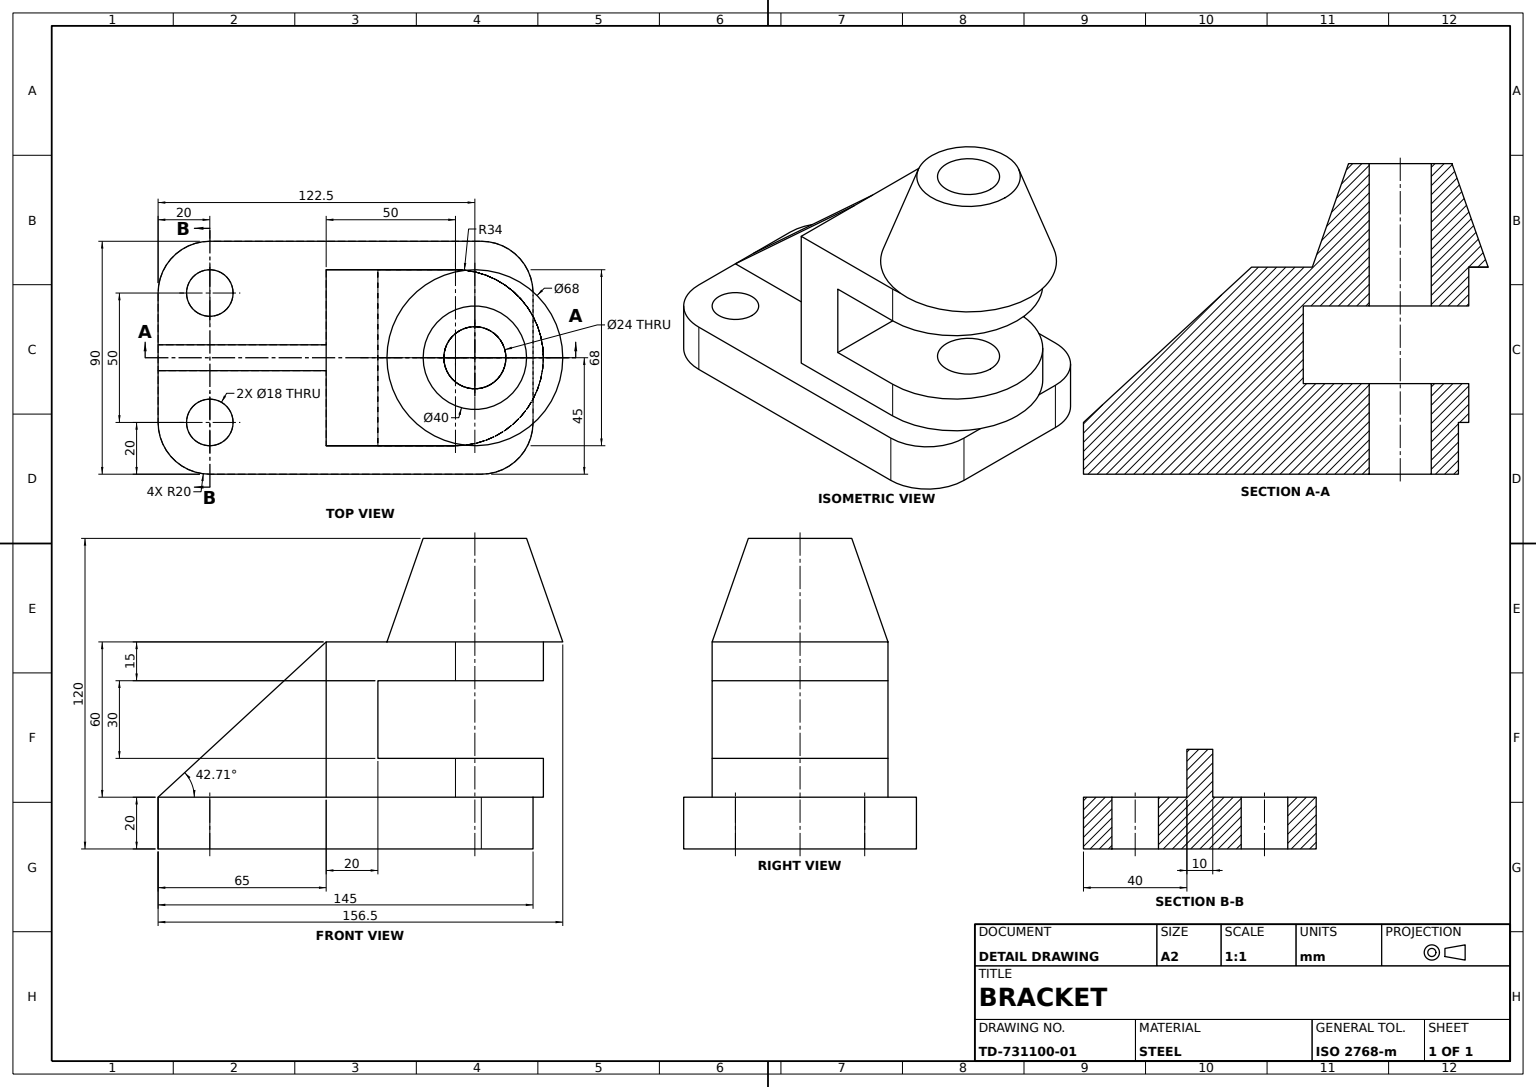
SolidWorks part; units mm, degrees
material "Plain Carbon Steel"
ref_plane "Front Plane" through (0, 0, 0) normal (0, 0, 1) x (1, 0, 0)
ref_plane "Top Plane" through (0, 0, 0) normal (0, 1, 0) x (1, 0, 0)
ref_plane "Right Plane" through (0, 0, 0) normal (1, 0, 0) x (0, 0, -1)
sketch "Base Plate Sketch" plane through (0, 0, 0) normal (0, 1, 0) x (1, 0, 0)
  line L0 (45, 0) -> (-45, 0) construction
  line L1 (-45, -72.5) -> (45, -72.5)
  line L2 (-45, -72.5) -> (-45, 72.5)
  line L3 (-45, 72.5) -> (45, 72.5)
  line L4 (45, -72.5) -> (45, 72.5)
  circle A0 centre (-25, -52.5) radius 9
  circle A1 centre (25, -52.5) radius 9
  point P11 (0, 0)
  dimension "D3" = 20
  dimension "D5" = 18
  dimension "D1" = 145
  dimension "D2" = 90
  dimension "D4" = 20
  dimension "D6" = 20
  dimension "D7" = 20
extrude "Base Plate" add sketch "Base Plate Sketch" along normal blind 20
fillet "Base Corner Fillets R20" radius 20 4 edges at (-45, 10, -72.5) (45, 10, -72.5) (-45, 10, 72.5) (45, 10, 72.5)
sketch "Upright Block Sketch" plane through (0, 20, 0) normal (0, 1, 0) x (1, 0, 0)
  line L0 (-34, -7.5) -> (34, -7.5)
  line L1 (34, -7.5) -> (34, 42.5)
  line L2 (-34, 42.5) -> (-34, -7.5)
  line L3 (-25, -72.5) -> (25, -72.5) construction
  arc A0 (34, 42.5) -> (-34, 42.5) centre (0, 42.5) ccw
  dimension "D1" = 68
  dimension "D2" = 50
  dimension "D3" = 65
extrude "Upright Block" add sketch "Upright Block Sketch" along normal blind 60
sketch "Side Slot Sketch" plane through (0, 80, 0) normal (0, 1, 0) x (1, 0, 0)
  line L0 (-34, 12.5) -> (34, 12.5)
  line L3 (-34, 42.5) -> (-34, -7.5)
  line L4 (-34, -7.5) -> (34, -7.5)
  line L5 (34, -7.5) -> (34, 42.5)
  line L6 (-34, 42.5) -> (-34, -7.5)
  line L7 (-34, -7.5) -> (34, -7.5)
  line L8 (34, -7.5) -> (34, 42.5)
  arc A1 (34, 42.5) -> (-34, 42.5) centre (0, 42.5) ccw
  arc A2 (34, 42.5) -> (-34, 42.5) centre (0, 42.5) ccw
  line M6 (-34, 42.5) -> (-34, -7.5)
  line M8 (34, -7.5) -> (34, 42.5)
  arc M9 (34, 42.5) -> (-34, 42.5) centre (0, 42.5) ccw
  dimension "D2" = 20
  dimension "D1" = 0
extrude "Side Slot" cut sketch "Side Slot Sketch" against normal blind 30 from offset 15 contours L0 M6 M8 M9 offset against normal yes
ref_plane "Plane1" through (0, 0, -50) normal (0, 0, 1) x (1, 0, 0)
sketch "Cone Boss Profile" plane through (0, 0, -50) normal (0, 0, 1) x (1, 0, 0)
  line L0 (0, 80) -> (0, 120)
  line L1 (-34, 80) -> (34, 80) construction
  line L2 (0, 120) -> (20, 120)
  line L3 (20, 120) -> (34, 80)
  line L4 (34, 80) -> (0, 80)
  dimension "D1" = 40
  dimension "D2" = 34
  dimension "D3" = 20
revolve "Cone Boss" add sketch "Cone Boss Profile" angle 360 about L0
sketch "Cone Bore Sketch" plane through (0, 120, 0) normal (0, 1, 0) x (1, 0, 0)
  circle A0 centre (0, 50) radius 12
  dimension "D1" = 24
extrude "Cone Bore Ø24" cut sketch "Cone Bore Sketch" against normal through all
sketch "Support Rib Sketch" plane through (0, 0, 0) normal (1, 0, 0) x (0, 0, -1)
  line L0 (-72.5, 20) -> (-7.5, 80)
rib "Support Rib 10mm" sketch "Support Rib Sketch" sketch "Support Rib Sketch" thickness 10 extrusion direction parallel to sketch draft on no parameters "D1"=10
